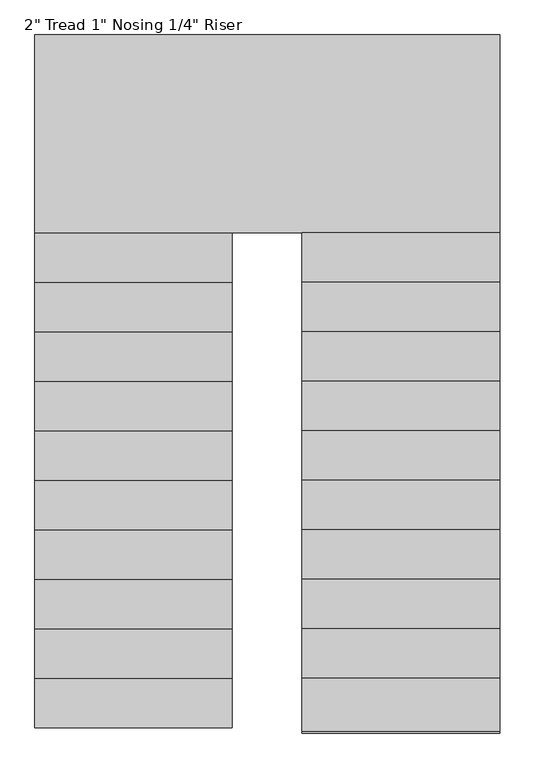
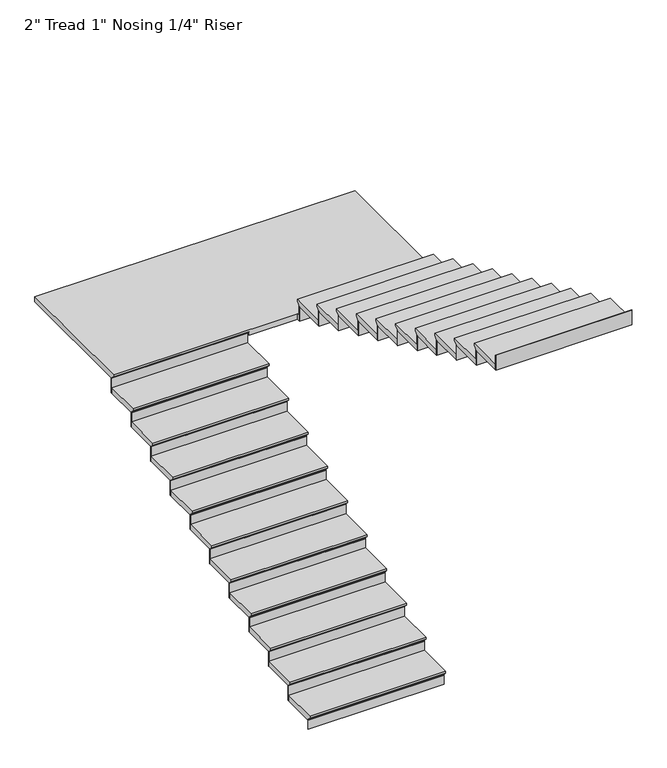
"""IFC4 building model written with IfcOpenShell, lengths in millimetres: stair flight geometry."""

from ifc_helpers import new_model, si_unit, origin, place, context, project, spatial, faceted_brep, source, transform, mapped, element, save


def stair_flight_66ca282f(model_context):
    return source(origin(), model_context, "Body", "Brep", [
        faceted_brep([(-629.5987998, 3364.6067329, 28923.0954545), (-629.5987998, 3364.6067329, 28942.1454545), (-1845.5417538, 3364.6067329, 28942.1454545), (-1845.5417538, 3364.6067329, 28923.0954545), (-629.5987998, 3390.0067329, 28897.6954545), (-1845.5417538, 3390.0067329, 28897.6954545), (-629.5987998, 3694.8067329, 28942.1454545), (-1845.5417538, 3694.8067329, 28942.1454545), (-1845.5417538, 3390.0067329, 28891.3454545), (-1845.5417538, 3694.8067329, 28891.3454545), (-629.5987998, 3694.8067329, 28891.3454545), (-629.5987998, 3390.0067329, 28891.3454545)], [[[0, 1, 2, 3]], [[4, 0, 3, 5]], [[2, 1, 6, 7]], [[8, 9, 10, 11]], [[2, 7, 9, 8, 5, 3]], [[8, 11, 4, 5]], [[6, 1, 0, 4, 11, 10]], [[7, 6, 10, 9]]]),
        faceted_brep([(-629.5987998, 3390.0067329, 28891.3454545), (-629.5987998, 3390.0067329, 28803.6), (-629.5987998, 3396.3567329, 28803.6), (-629.5987998, 3396.3567329, 28891.3454545), (-1845.5417538, 3390.0067329, 28891.3454545), (-1845.5417538, 3396.3567329, 28891.3454545), (-1845.5417538, 3396.3567329, 28803.6), (-1845.5417538, 3390.0067329, 28803.6)], [[[0, 1, 2, 3]], [[4, 5, 6, 7]], [[1, 0, 4, 7]], [[2, 1, 7, 6]], [[3, 2, 6, 5]], [[0, 3, 5, 4]]]),
        faceted_brep([(-629.5987998, 3694.8067329, 29029.8909091), (-629.5987998, 3694.8067329, 28891.3454545), (-629.5987998, 3701.1567329, 28891.3454545), (-629.5987998, 3701.1567329, 29029.8909091), (-1845.5417538, 3694.8067329, 29029.8909091), (-1845.5417538, 3701.1567329, 29029.8909091), (-1845.5417538, 3701.1567329, 28891.3454545), (-1845.5417538, 3694.8067329, 28891.3454545)], [[[0, 1, 2, 3]], [[4, 5, 6, 7]], [[1, 0, 4, 7]], [[2, 1, 7, 6]], [[3, 2, 6, 5]], [[0, 3, 5, 4]]]),
        faceted_brep([(-1845.5417538, 3669.4067329, 29080.6909091), (-629.5987998, 3669.4067329, 29080.6909091), (-629.5987998, 3999.6067329, 29080.6909091), (-1845.5417538, 3999.6067329, 29080.6909091), (-1845.5417538, 3694.8067329, 29029.8909091), (-1845.5417538, 3999.6067329, 29029.8909091), (-629.5987998, 3999.6067329, 29029.8909091), (-629.5987998, 3694.8067329, 29029.8909091), (-1845.5417538, 3694.8067329, 29036.2409091), (-1845.5417538, 3669.4067329, 29061.6409091), (-629.5987998, 3694.8067329, 29036.2409091), (-629.5987998, 3669.4067329, 29061.6409091)], [[[0, 1, 2, 3]], [[4, 5, 6, 7]], [[0, 3, 5, 4, 8, 9]], [[4, 7, 10, 8]], [[2, 1, 11, 10, 7, 6]], [[3, 2, 6, 5]], [[11, 1, 0, 9]], [[10, 11, 9, 8]]]),
        faceted_brep([(-629.5987998, 3999.6067329, 29168.4363636), (-629.5987998, 3999.6067329, 29029.8909091), (-629.5987998, 4005.9567329, 29029.8909091), (-629.5987998, 4005.9567329, 29168.4363636), (-1845.5417538, 3999.6067329, 29168.4363636), (-1845.5417538, 4005.9567329, 29168.4363636), (-1845.5417538, 4005.9567329, 29029.8909091), (-1845.5417538, 3999.6067329, 29029.8909091)], [[[0, 1, 2, 3]], [[4, 5, 6, 7]], [[1, 0, 4, 7]], [[2, 1, 7, 6]], [[3, 2, 6, 5]], [[0, 3, 5, 4]]]),
        faceted_brep([(-1845.5417538, 3974.2067329, 29219.2363636), (-629.5987998, 3974.2067329, 29219.2363636), (-629.5987998, 4304.4067329, 29219.2363636), (-1845.5417538, 4304.4067329, 29219.2363636), (-1845.5417538, 3999.6067329, 29168.4363636), (-1845.5417538, 4304.4067329, 29168.4363636), (-629.5987998, 4304.4067329, 29168.4363636), (-629.5987998, 3999.6067329, 29168.4363636), (-1845.5417538, 3999.6067329, 29174.7863636), (-1845.5417538, 3974.2067329, 29200.1863636), (-629.5987998, 3999.6067329, 29174.7863636), (-629.5987998, 3974.2067329, 29200.1863636)], [[[0, 1, 2, 3]], [[4, 5, 6, 7]], [[0, 3, 5, 4, 8, 9]], [[4, 7, 10, 8]], [[2, 1, 11, 10, 7, 6]], [[3, 2, 6, 5]], [[11, 1, 0, 9]], [[10, 11, 9, 8]]]),
        faceted_brep([(-629.5987998, 4304.4067329, 29306.9818182), (-629.5987998, 4304.4067329, 29168.4363636), (-629.5987998, 4310.7567329, 29168.4363636), (-629.5987998, 4310.7567329, 29306.9818182), (-1845.5417538, 4304.4067329, 29306.9818182), (-1845.5417538, 4310.7567329, 29306.9818182), (-1845.5417538, 4310.7567329, 29168.4363636), (-1845.5417538, 4304.4067329, 29168.4363636)], [[[0, 1, 2, 3]], [[4, 5, 6, 7]], [[1, 0, 4, 7]], [[2, 1, 7, 6]], [[3, 2, 6, 5]], [[0, 3, 5, 4]]]),
        faceted_brep([(-1845.5417538, 4279.0067329, 29357.7818182), (-629.5987998, 4279.0067329, 29357.7818182), (-629.5987998, 4609.2067329, 29357.7818182), (-1845.5417538, 4609.2067329, 29357.7818182), (-1845.5417538, 4304.4067329, 29306.9818182), (-1845.5417538, 4609.2067329, 29306.9818182), (-629.5987998, 4609.2067329, 29306.9818182), (-629.5987998, 4304.4067329, 29306.9818182), (-1845.5417538, 4304.4067329, 29313.3318182), (-1845.5417538, 4279.0067329, 29338.7318182), (-629.5987998, 4304.4067329, 29313.3318182), (-629.5987998, 4279.0067329, 29338.7318182)], [[[0, 1, 2, 3]], [[4, 5, 6, 7]], [[0, 3, 5, 4, 8, 9]], [[4, 7, 10, 8]], [[2, 1, 11, 10, 7, 6]], [[3, 2, 6, 5]], [[11, 1, 0, 9]], [[10, 11, 9, 8]]]),
        faceted_brep([(-629.5987998, 4609.2067329, 29445.5272727), (-629.5987998, 4609.2067329, 29306.9818182), (-629.5987998, 4615.5567329, 29306.9818182), (-629.5987998, 4615.5567329, 29445.5272727), (-1845.5417538, 4609.2067329, 29445.5272727), (-1845.5417538, 4615.5567329, 29445.5272727), (-1845.5417538, 4615.5567329, 29306.9818182), (-1845.5417538, 4609.2067329, 29306.9818182)], [[[0, 1, 2, 3]], [[4, 5, 6, 7]], [[1, 0, 4, 7]], [[2, 1, 7, 6]], [[3, 2, 6, 5]], [[0, 3, 5, 4]]]),
        faceted_brep([(-1845.5417538, 4583.8067329, 29496.3272727), (-629.5987998, 4583.8067329, 29496.3272727), (-629.5987998, 4914.0067329, 29496.3272727), (-1845.5417538, 4914.0067329, 29496.3272727), (-1845.5417538, 4609.2067329, 29445.5272727), (-1845.5417538, 4914.0067329, 29445.5272727), (-629.5987998, 4914.0067329, 29445.5272727), (-629.5987998, 4609.2067329, 29445.5272727), (-1845.5417538, 4609.2067329, 29451.8772727), (-1845.5417538, 4583.8067329, 29477.2772727), (-629.5987998, 4609.2067329, 29451.8772727), (-629.5987998, 4583.8067329, 29477.2772727)], [[[0, 1, 2, 3]], [[4, 5, 6, 7]], [[0, 3, 5, 4, 8, 9]], [[4, 7, 10, 8]], [[2, 1, 11, 10, 7, 6]], [[3, 2, 6, 5]], [[11, 1, 0, 9]], [[10, 11, 9, 8]]]),
        faceted_brep([(-629.5987998, 4914.0067329, 29584.0727273), (-629.5987998, 4914.0067329, 29445.5272727), (-629.5987998, 4920.3567329, 29445.5272727), (-629.5987998, 4920.3567329, 29584.0727273), (-1845.5417538, 4914.0067329, 29584.0727273), (-1845.5417538, 4920.3567329, 29584.0727273), (-1845.5417538, 4920.3567329, 29445.5272727), (-1845.5417538, 4914.0067329, 29445.5272727)], [[[0, 1, 2, 3]], [[4, 5, 6, 7]], [[1, 0, 4, 7]], [[2, 1, 7, 6]], [[3, 2, 6, 5]], [[0, 3, 5, 4]]]),
        faceted_brep([(-1845.5417538, 4888.6067329, 29634.8727273), (-629.5987998, 4888.6067329, 29634.8727273), (-629.5987998, 5218.8067329, 29634.8727273), (-1845.5417538, 5218.8067329, 29634.8727273), (-1845.5417538, 4914.0067329, 29584.0727273), (-1845.5417538, 5218.8067329, 29584.0727273), (-629.5987998, 5218.8067329, 29584.0727273), (-629.5987998, 4914.0067329, 29584.0727273), (-1845.5417538, 4914.0067329, 29590.4227273), (-1845.5417538, 4888.6067329, 29615.8227273), (-629.5987998, 4914.0067329, 29590.4227273), (-629.5987998, 4888.6067329, 29615.8227273)], [[[0, 1, 2, 3]], [[4, 5, 6, 7]], [[0, 3, 5, 4, 8, 9]], [[4, 7, 10, 8]], [[2, 1, 11, 10, 7, 6]], [[3, 2, 6, 5]], [[11, 1, 0, 9]], [[10, 11, 9, 8]]]),
        faceted_brep([(-629.5987998, 5218.8067329, 29722.6181818), (-629.5987998, 5218.8067329, 29584.0727273), (-629.5987998, 5225.1567329, 29584.0727273), (-629.5987998, 5225.1567329, 29722.6181818), (-1845.5417538, 5218.8067329, 29722.6181818), (-1845.5417538, 5225.1567329, 29722.6181818), (-1845.5417538, 5225.1567329, 29584.0727273), (-1845.5417538, 5218.8067329, 29584.0727273)], [[[0, 1, 2, 3]], [[4, 5, 6, 7]], [[1, 0, 4, 7]], [[2, 1, 7, 6]], [[3, 2, 6, 5]], [[0, 3, 5, 4]]]),
        faceted_brep([(-1845.5417538, 5193.4067329, 29773.4181818), (-629.5987998, 5193.4067329, 29773.4181818), (-629.5987998, 5523.6067329, 29773.4181818), (-1845.5417538, 5523.6067329, 29773.4181818), (-1845.5417538, 5218.8067329, 29722.6181818), (-1845.5417538, 5523.6067329, 29722.6181818), (-629.5987998, 5523.6067329, 29722.6181818), (-629.5987998, 5218.8067329, 29722.6181818), (-1845.5417538, 5218.8067329, 29728.9681818), (-1845.5417538, 5193.4067329, 29754.3681818), (-629.5987998, 5218.8067329, 29728.9681818), (-629.5987998, 5193.4067329, 29754.3681818)], [[[0, 1, 2, 3]], [[4, 5, 6, 7]], [[0, 3, 5, 4, 8, 9]], [[4, 7, 10, 8]], [[2, 1, 11, 10, 7, 6]], [[3, 2, 6, 5]], [[11, 1, 0, 9]], [[10, 11, 9, 8]]]),
        faceted_brep([(-629.5987998, 5523.6067329, 29861.1636364), (-629.5987998, 5523.6067329, 29722.6181818), (-629.5987998, 5529.9567329, 29722.6181818), (-629.5987998, 5529.9567329, 29861.1636364), (-1845.5417538, 5523.6067329, 29861.1636364), (-1845.5417538, 5529.9567329, 29861.1636364), (-1845.5417538, 5529.9567329, 29722.6181818), (-1845.5417538, 5523.6067329, 29722.6181818)], [[[0, 1, 2, 3]], [[4, 5, 6, 7]], [[1, 0, 4, 7]], [[2, 1, 7, 6]], [[3, 2, 6, 5]], [[0, 3, 5, 4]]]),
        faceted_brep([(-1845.5417538, 5498.2067329, 29911.9636364), (-629.5987998, 5498.2067329, 29911.9636364), (-629.5987998, 5828.4067329, 29911.9636364), (-1845.5417538, 5828.4067329, 29911.9636364), (-1845.5417538, 5523.6067329, 29861.1636364), (-1845.5417538, 5828.4067329, 29861.1636364), (-629.5987998, 5828.4067329, 29861.1636364), (-629.5987998, 5523.6067329, 29861.1636364), (-1845.5417538, 5523.6067329, 29867.5136364), (-1845.5417538, 5498.2067329, 29892.9136364), (-629.5987998, 5523.6067329, 29867.5136364), (-629.5987998, 5498.2067329, 29892.9136364)], [[[0, 1, 2, 3]], [[4, 5, 6, 7]], [[0, 3, 5, 4, 8, 9]], [[4, 7, 10, 8]], [[2, 1, 11, 10, 7, 6]], [[3, 2, 6, 5]], [[11, 1, 0, 9]], [[10, 11, 9, 8]]]),
        faceted_brep([(-629.5987998, 5828.4067329, 29999.7090909), (-629.5987998, 5828.4067329, 29861.1636364), (-629.5987998, 5834.7567329, 29861.1636364), (-629.5987998, 5834.7567329, 29999.7090909), (-1845.5417538, 5828.4067329, 29999.7090909), (-1845.5417538, 5834.7567329, 29999.7090909), (-1845.5417538, 5834.7567329, 29861.1636364), (-1845.5417538, 5828.4067329, 29861.1636364)], [[[0, 1, 2, 3]], [[4, 5, 6, 7]], [[1, 0, 4, 7]], [[2, 1, 7, 6]], [[3, 2, 6, 5]], [[0, 3, 5, 4]]]),
        faceted_brep([(-1845.5417538, 5803.0067329, 30050.5090909), (-629.5987998, 5803.0067329, 30050.5090909), (-629.5987998, 6133.2067329, 30050.5090909), (-1845.5417538, 6133.2067329, 30050.5090909), (-1845.5417538, 5828.4067329, 29999.7090909), (-1845.5417538, 6133.2067329, 29999.7090909), (-629.5987998, 6133.2067329, 29999.7090909), (-629.5987998, 5828.4067329, 29999.7090909), (-1845.5417538, 5828.4067329, 30006.0590909), (-1845.5417538, 5803.0067329, 30031.4590909), (-629.5987998, 5828.4067329, 30006.0590909), (-629.5987998, 5803.0067329, 30031.4590909)], [[[0, 1, 2, 3]], [[4, 5, 6, 7]], [[0, 3, 5, 4, 8, 9]], [[4, 7, 10, 8]], [[2, 1, 11, 10, 7, 6]], [[3, 2, 6, 5]], [[11, 1, 0, 9]], [[10, 11, 9, 8]]]),
        faceted_brep([(-629.5987998, 6133.2067329, 30138.2545455), (-629.5987998, 6133.2067329, 29999.7090909), (-629.5987998, 6139.5567329, 29999.7090909), (-629.5987998, 6139.5567329, 30138.2545455), (-1845.5417538, 6133.2067329, 30138.2545455), (-1845.5417538, 6139.5567329, 30138.2545455), (-1845.5417538, 6139.5567329, 29999.7090909), (-1845.5417538, 6133.2067329, 29999.7090909)], [[[0, 1, 2, 3]], [[4, 5, 6, 7]], [[1, 0, 4, 7]], [[2, 1, 7, 6]], [[3, 2, 6, 5]], [[0, 3, 5, 4]]]),
        faceted_brep([(-1845.5417538, 6107.8067329, 30189.0545455), (-629.5987998, 6107.8067329, 30189.0545455), (-629.5987998, 6438.0067329, 30189.0545455), (-1845.5417538, 6438.0067329, 30189.0545455), (-1845.5417538, 6133.2067329, 30138.2545455), (-1845.5417538, 6438.0067329, 30138.2545455), (-629.5987998, 6438.0067329, 30138.2545455), (-629.5987998, 6133.2067329, 30138.2545455), (-1845.5417538, 6133.2067329, 30144.6045455), (-1845.5417538, 6107.8067329, 30170.0045455), (-629.5987998, 6133.2067329, 30144.6045455), (-629.5987998, 6107.8067329, 30170.0045455)], [[[0, 1, 2, 3]], [[4, 5, 6, 7]], [[0, 3, 5, 4, 8, 9]], [[4, 7, 10, 8]], [[2, 1, 11, 10, 7, 6]], [[3, 2, 6, 5]], [[11, 1, 0, 9]], [[10, 11, 9, 8]]]),
        faceted_brep([(-629.5987998, 6438.0067329, 30276.8), (-629.5987998, 6438.0067329, 30138.2545455), (-629.5987998, 6444.3567329, 30138.2545455), (-629.5987998, 6444.3567329, 30276.8), (-1845.5417538, 6438.0067329, 30276.8), (-1845.5417538, 6444.3567329, 30276.8), (-1845.5417538, 6444.3567329, 30138.2545455), (-1845.5417538, 6438.0067329, 30138.2545455)], [[[0, 1, 2, 3]], [[4, 5, 6, 7]], [[1, 0, 4, 7]], [[2, 1, 7, 6]], [[3, 2, 6, 5]], [[0, 3, 5, 4]]]),
        faceted_brep([(1021.4012085, 6387.2067329, 30327.6), (1021.4012085, 7631.8067329, 30327.6), (-1845.5417538, 7631.8067329, 30327.6), (-1845.5417538, 6412.6067329, 30327.6), (-197.7987915, 6412.6067329, 30327.6), (-197.7987915, 6387.2067329, 30327.6), (1021.4012085, 7631.8067329, 30276.8), (1021.4012085, 6387.2067329, 30276.8), (-197.7987915, 6387.2067329, 30276.8), (-197.7987915, 6412.6067329, 30276.8), (-629.5987998, 6412.6067329, 30276.8), (-629.5987998, 6438.0067329, 30276.8), (-1845.5417538, 6438.0067329, 30276.8), (-1845.5417538, 7631.8067329, 30276.8), (-629.5987998, 6438.0067329, 30283.15), (-1845.5417538, 6438.0067329, 30283.15), (-1845.5417538, 6412.6067329, 30308.55), (-629.5987998, 6412.6067329, 30308.55)], [[[0, 1, 2, 3, 4, 5]], [[6, 7, 8, 9, 10, 11, 12, 13]], [[1, 0, 7, 6]], [[2, 1, 6, 13]], [[12, 11, 14, 15]], [[4, 3, 16, 17, 10, 9]], [[5, 4, 9, 8]], [[0, 5, 8, 7]], [[16, 15, 14, 17]], [[3, 2, 13, 12, 15, 16]], [[11, 10, 17, 14]]]),
        faceted_brep([(-197.7987915, 6387.2067329, 30415.3454545), (-197.7987915, 6387.2067329, 30276.8), (-197.7987915, 6380.8567329, 30276.8), (-197.7987915, 6380.8567329, 30415.3454545), (1021.4012085, 6387.2067329, 30415.3454545), (1021.4012085, 6380.8567329, 30415.3454545), (1021.4012085, 6380.8567329, 30276.8), (1021.4012085, 6387.2067329, 30276.8)], [[[0, 1, 2, 3]], [[4, 5, 6, 7]], [[1, 0, 4, 7]], [[2, 1, 7, 6]], [[3, 2, 6, 5]], [[0, 3, 5, 4]]]),
        faceted_brep([(1021.4012085, 6412.6067329, 30466.1454545), (-197.7987915, 6412.6067329, 30466.1454545), (-197.7987915, 6082.4067329, 30466.1454545), (1021.4012085, 6082.4067329, 30466.1454545), (1021.4012085, 6387.2067329, 30415.3454545), (1021.4012085, 6082.4067329, 30415.3454545), (-197.7987915, 6082.4067329, 30415.3454545), (-197.7987915, 6387.2067329, 30415.3454545), (1021.4012085, 6387.2067329, 30421.6954545), (1021.4012085, 6412.6067329, 30447.0954545), (-197.7987915, 6387.2067329, 30421.6954545), (-197.7987915, 6412.6067329, 30447.0954545)], [[[0, 1, 2, 3]], [[4, 5, 6, 7]], [[0, 3, 5, 4, 8, 9]], [[4, 7, 10, 8]], [[2, 1, 11, 10, 7, 6]], [[3, 2, 6, 5]], [[11, 1, 0, 9]], [[10, 11, 9, 8]]]),
        faceted_brep([(-197.7987915, 6082.4067329, 30553.8909091), (-197.7987915, 6082.4067329, 30415.3454545), (-197.7987915, 6076.0567329, 30415.3454545), (-197.7987915, 6076.0567329, 30553.8909091), (1021.4012085, 6082.4067329, 30553.8909091), (1021.4012085, 6076.0567329, 30553.8909091), (1021.4012085, 6076.0567329, 30415.3454545), (1021.4012085, 6082.4067329, 30415.3454545)], [[[0, 1, 2, 3]], [[4, 5, 6, 7]], [[1, 0, 4, 7]], [[2, 1, 7, 6]], [[3, 2, 6, 5]], [[0, 3, 5, 4]]]),
        faceted_brep([(1021.4012085, 6107.8067329, 30604.6909091), (-197.7987915, 6107.8067329, 30604.6909091), (-197.7987915, 5777.6067329, 30604.6909091), (1021.4012085, 5777.6067329, 30604.6909091), (1021.4012085, 6082.4067329, 30553.8909091), (1021.4012085, 5777.6067329, 30553.8909091), (-197.7987915, 5777.6067329, 30553.8909091), (-197.7987915, 6082.4067329, 30553.8909091), (1021.4012085, 6082.4067329, 30560.2409091), (1021.4012085, 6107.8067329, 30585.6409091), (-197.7987915, 6082.4067329, 30560.2409091), (-197.7987915, 6107.8067329, 30585.6409091)], [[[0, 1, 2, 3]], [[4, 5, 6, 7]], [[0, 3, 5, 4, 8, 9]], [[4, 7, 10, 8]], [[2, 1, 11, 10, 7, 6]], [[3, 2, 6, 5]], [[11, 1, 0, 9]], [[10, 11, 9, 8]]]),
        faceted_brep([(-197.7987915, 5777.6067329, 30692.4363636), (-197.7987915, 5777.6067329, 30553.8909091), (-197.7987915, 5771.2567329, 30553.8909091), (-197.7987915, 5771.2567329, 30692.4363636), (1021.4012085, 5777.6067329, 30692.4363636), (1021.4012085, 5771.2567329, 30692.4363636), (1021.4012085, 5771.2567329, 30553.8909091), (1021.4012085, 5777.6067329, 30553.8909091)], [[[0, 1, 2, 3]], [[4, 5, 6, 7]], [[1, 0, 4, 7]], [[2, 1, 7, 6]], [[3, 2, 6, 5]], [[0, 3, 5, 4]]]),
        faceted_brep([(1021.4012085, 5803.0067329, 30743.2363636), (-197.7987915, 5803.0067329, 30743.2363636), (-197.7987915, 5472.8067329, 30743.2363636), (1021.4012085, 5472.8067329, 30743.2363636), (1021.4012085, 5777.6067329, 30692.4363636), (1021.4012085, 5472.8067329, 30692.4363636), (-197.7987915, 5472.8067329, 30692.4363636), (-197.7987915, 5777.6067329, 30692.4363636), (1021.4012085, 5777.6067329, 30698.7863636), (1021.4012085, 5803.0067329, 30724.1863636), (-197.7987915, 5777.6067329, 30698.7863636), (-197.7987915, 5803.0067329, 30724.1863636)], [[[0, 1, 2, 3]], [[4, 5, 6, 7]], [[0, 3, 5, 4, 8, 9]], [[4, 7, 10, 8]], [[2, 1, 11, 10, 7, 6]], [[3, 2, 6, 5]], [[11, 1, 0, 9]], [[10, 11, 9, 8]]]),
        faceted_brep([(-197.7987915, 5472.8067329, 30830.9818182), (-197.7987915, 5472.8067329, 30692.4363636), (-197.7987915, 5466.4567329, 30692.4363636), (-197.7987915, 5466.4567329, 30830.9818182), (1021.4012085, 5472.8067329, 30830.9818182), (1021.4012085, 5466.4567329, 30830.9818182), (1021.4012085, 5466.4567329, 30692.4363636), (1021.4012085, 5472.8067329, 30692.4363636)], [[[0, 1, 2, 3]], [[4, 5, 6, 7]], [[1, 0, 4, 7]], [[2, 1, 7, 6]], [[3, 2, 6, 5]], [[0, 3, 5, 4]]]),
        faceted_brep([(1021.4012085, 5498.2067329, 30881.7818182), (-197.7987915, 5498.2067329, 30881.7818182), (-197.7987915, 5168.0067329, 30881.7818182), (1021.4012085, 5168.0067329, 30881.7818182), (1021.4012085, 5472.8067329, 30830.9818182), (1021.4012085, 5168.0067329, 30830.9818182), (-197.7987915, 5168.0067329, 30830.9818182), (-197.7987915, 5472.8067329, 30830.9818182), (1021.4012085, 5472.8067329, 30837.3318182), (1021.4012085, 5498.2067329, 30862.7318182), (-197.7987915, 5472.8067329, 30837.3318182), (-197.7987915, 5498.2067329, 30862.7318182)], [[[0, 1, 2, 3]], [[4, 5, 6, 7]], [[0, 3, 5, 4, 8, 9]], [[4, 7, 10, 8]], [[2, 1, 11, 10, 7, 6]], [[3, 2, 6, 5]], [[11, 1, 0, 9]], [[10, 11, 9, 8]]]),
        faceted_brep([(-197.7987915, 5168.0067329, 30969.5272727), (-197.7987915, 5168.0067329, 30830.9818182), (-197.7987915, 5161.6567329, 30830.9818182), (-197.7987915, 5161.6567329, 30969.5272727), (1021.4012085, 5168.0067329, 30969.5272727), (1021.4012085, 5161.6567329, 30969.5272727), (1021.4012085, 5161.6567329, 30830.9818182), (1021.4012085, 5168.0067329, 30830.9818182)], [[[0, 1, 2, 3]], [[4, 5, 6, 7]], [[1, 0, 4, 7]], [[2, 1, 7, 6]], [[3, 2, 6, 5]], [[0, 3, 5, 4]]]),
        faceted_brep([(1021.4012085, 5193.4067329, 31020.3272727), (-197.7987915, 5193.4067329, 31020.3272727), (-197.7987915, 4863.2067329, 31020.3272727), (1021.4012085, 4863.2067329, 31020.3272727), (1021.4012085, 5168.0067329, 30969.5272727), (1021.4012085, 4863.2067329, 30969.5272727), (-197.7987915, 4863.2067329, 30969.5272727), (-197.7987915, 5168.0067329, 30969.5272727), (1021.4012085, 5168.0067329, 30975.8772727), (1021.4012085, 5193.4067329, 31001.2772727), (-197.7987915, 5168.0067329, 30975.8772727), (-197.7987915, 5193.4067329, 31001.2772727)], [[[0, 1, 2, 3]], [[4, 5, 6, 7]], [[0, 3, 5, 4, 8, 9]], [[4, 7, 10, 8]], [[2, 1, 11, 10, 7, 6]], [[3, 2, 6, 5]], [[11, 1, 0, 9]], [[10, 11, 9, 8]]]),
        faceted_brep([(-197.7987915, 4863.2067329, 31108.0727273), (-197.7987915, 4863.2067329, 30969.5272727), (-197.7987915, 4856.8567329, 30969.5272727), (-197.7987915, 4856.8567329, 31108.0727273), (1021.4012085, 4863.2067329, 31108.0727273), (1021.4012085, 4856.8567329, 31108.0727273), (1021.4012085, 4856.8567329, 30969.5272727), (1021.4012085, 4863.2067329, 30969.5272727)], [[[0, 1, 2, 3]], [[4, 5, 6, 7]], [[1, 0, 4, 7]], [[2, 1, 7, 6]], [[3, 2, 6, 5]], [[0, 3, 5, 4]]]),
        faceted_brep([(1021.4012085, 4888.6067329, 31158.8727273), (-197.7987915, 4888.6067329, 31158.8727273), (-197.7987915, 4558.4067329, 31158.8727273), (1021.4012085, 4558.4067329, 31158.8727273), (1021.4012085, 4863.2067329, 31108.0727273), (1021.4012085, 4558.4067329, 31108.0727273), (-197.7987915, 4558.4067329, 31108.0727273), (-197.7987915, 4863.2067329, 31108.0727273), (1021.4012085, 4863.2067329, 31114.4227273), (1021.4012085, 4888.6067329, 31139.8227273), (-197.7987915, 4863.2067329, 31114.4227273), (-197.7987915, 4888.6067329, 31139.8227273)], [[[0, 1, 2, 3]], [[4, 5, 6, 7]], [[0, 3, 5, 4, 8, 9]], [[4, 7, 10, 8]], [[2, 1, 11, 10, 7, 6]], [[3, 2, 6, 5]], [[11, 1, 0, 9]], [[10, 11, 9, 8]]]),
        faceted_brep([(-197.7987915, 4558.4067329, 31246.6181818), (-197.7987915, 4558.4067329, 31108.0727273), (-197.7987915, 4552.0567329, 31108.0727273), (-197.7987915, 4552.0567329, 31246.6181818), (1021.4012085, 4558.4067329, 31246.6181818), (1021.4012085, 4552.0567329, 31246.6181818), (1021.4012085, 4552.0567329, 31108.0727273), (1021.4012085, 4558.4067329, 31108.0727273)], [[[0, 1, 2, 3]], [[4, 5, 6, 7]], [[1, 0, 4, 7]], [[2, 1, 7, 6]], [[3, 2, 6, 5]], [[0, 3, 5, 4]]]),
        faceted_brep([(1021.4012085, 4583.8067329, 31297.4181818), (-197.7987915, 4583.8067329, 31297.4181818), (-197.7987915, 4253.6067329, 31297.4181818), (1021.4012085, 4253.6067329, 31297.4181818), (1021.4012085, 4558.4067329, 31246.6181818), (1021.4012085, 4253.6067329, 31246.6181818), (-197.7987915, 4253.6067329, 31246.6181818), (-197.7987915, 4558.4067329, 31246.6181818), (1021.4012085, 4558.4067329, 31252.9681818), (1021.4012085, 4583.8067329, 31278.3681818), (-197.7987915, 4558.4067329, 31252.9681818), (-197.7987915, 4583.8067329, 31278.3681818)], [[[0, 1, 2, 3]], [[4, 5, 6, 7]], [[0, 3, 5, 4, 8, 9]], [[4, 7, 10, 8]], [[2, 1, 11, 10, 7, 6]], [[3, 2, 6, 5]], [[11, 1, 0, 9]], [[10, 11, 9, 8]]]),
        faceted_brep([(-197.7987915, 4253.6067329, 31385.1636364), (-197.7987915, 4253.6067329, 31246.6181818), (-197.7987915, 4247.2567329, 31246.6181818), (-197.7987915, 4247.2567329, 31385.1636364), (1021.4012085, 4253.6067329, 31385.1636364), (1021.4012085, 4247.2567329, 31385.1636364), (1021.4012085, 4247.2567329, 31246.6181818), (1021.4012085, 4253.6067329, 31246.6181818)], [[[0, 1, 2, 3]], [[4, 5, 6, 7]], [[1, 0, 4, 7]], [[2, 1, 7, 6]], [[3, 2, 6, 5]], [[0, 3, 5, 4]]]),
        faceted_brep([(1021.4012085, 4279.0067329, 31435.9636364), (-197.7987915, 4279.0067329, 31435.9636364), (-197.7987915, 3948.8067329, 31435.9636364), (1021.4012085, 3948.8067329, 31435.9636364), (1021.4012085, 4253.6067329, 31385.1636364), (1021.4012085, 3948.8067329, 31385.1636364), (-197.7987915, 3948.8067329, 31385.1636364), (-197.7987915, 4253.6067329, 31385.1636364), (1021.4012085, 4253.6067329, 31391.5136364), (1021.4012085, 4279.0067329, 31416.9136364), (-197.7987915, 4253.6067329, 31391.5136364), (-197.7987915, 4279.0067329, 31416.9136364)], [[[0, 1, 2, 3]], [[4, 5, 6, 7]], [[0, 3, 5, 4, 8, 9]], [[4, 7, 10, 8]], [[2, 1, 11, 10, 7, 6]], [[3, 2, 6, 5]], [[11, 1, 0, 9]], [[10, 11, 9, 8]]]),
        faceted_brep([(-197.7987915, 3948.8067329, 31523.7090909), (-197.7987915, 3948.8067329, 31385.1636364), (-197.7987915, 3942.4567329, 31385.1636364), (-197.7987915, 3942.4567329, 31523.7090909), (1021.4012085, 3948.8067329, 31523.7090909), (1021.4012085, 3942.4567329, 31523.7090909), (1021.4012085, 3942.4567329, 31385.1636364), (1021.4012085, 3948.8067329, 31385.1636364)], [[[0, 1, 2, 3]], [[4, 5, 6, 7]], [[1, 0, 4, 7]], [[2, 1, 7, 6]], [[3, 2, 6, 5]], [[0, 3, 5, 4]]]),
        faceted_brep([(1021.4012085, 3974.2067329, 31574.5090909), (-197.7987915, 3974.2067329, 31574.5090909), (-197.7987915, 3644.0067329, 31574.5090909), (1021.4012085, 3644.0067329, 31574.5090909), (1021.4012085, 3948.8067329, 31523.7090909), (1021.4012085, 3644.0067329, 31523.7090909), (-197.7987915, 3644.0067329, 31523.7090909), (-197.7987915, 3948.8067329, 31523.7090909), (1021.4012085, 3948.8067329, 31530.0590909), (1021.4012085, 3974.2067329, 31555.4590909), (-197.7987915, 3948.8067329, 31530.0590909), (-197.7987915, 3974.2067329, 31555.4590909)], [[[0, 1, 2, 3]], [[4, 5, 6, 7]], [[0, 3, 5, 4, 8, 9]], [[4, 7, 10, 8]], [[2, 1, 11, 10, 7, 6]], [[3, 2, 6, 5]], [[11, 1, 0, 9]], [[10, 11, 9, 8]]]),
        faceted_brep([(-197.7987915, 3644.0067329, 31662.2545455), (-197.7987915, 3644.0067329, 31523.7090909), (-197.7987915, 3637.6567329, 31523.7090909), (-197.7987915, 3637.6567329, 31662.2545455), (1021.4012085, 3644.0067329, 31662.2545455), (1021.4012085, 3637.6567329, 31662.2545455), (1021.4012085, 3637.6567329, 31523.7090909), (1021.4012085, 3644.0067329, 31523.7090909)], [[[0, 1, 2, 3]], [[4, 5, 6, 7]], [[1, 0, 4, 7]], [[2, 1, 7, 6]], [[3, 2, 6, 5]], [[0, 3, 5, 4]]]),
        faceted_brep([(-197.7987915, 3339.2067329, 31800.8), (-197.7987915, 3339.2067329, 31662.2545455), (-197.7987915, 3332.8567329, 31662.2545455), (-197.7987915, 3332.8567329, 31800.8), (1021.4012085, 3339.2067329, 31800.8), (1021.4012085, 3332.8567329, 31800.8), (1021.4012085, 3332.8567329, 31662.2545455), (1021.4012085, 3339.2067329, 31662.2545455)], [[[0, 1, 2, 3]], [[4, 5, 6, 7]], [[1, 0, 4, 7]], [[2, 1, 7, 6]], [[3, 2, 6, 5]], [[0, 3, 5, 4]]]),
        faceted_brep([(1021.4012085, 3669.4067329, 31713.0545455), (-197.7987915, 3669.4067329, 31713.0545455), (-197.7987915, 3339.2067329, 31713.0545455), (1021.4012085, 3339.2067329, 31713.0545455), (1021.4012085, 3644.0067329, 31662.2545455), (1021.4012085, 3339.2067329, 31662.2545455), (-197.7987915, 3339.2067329, 31662.2545455), (-197.7987915, 3644.0067329, 31662.2545455), (1021.4012085, 3644.0067329, 31668.6045455), (1021.4012085, 3669.4067329, 31694.0045455), (-197.7987915, 3644.0067329, 31668.6045455), (-197.7987915, 3669.4067329, 31694.0045455)], [[[0, 1, 2, 3]], [[4, 5, 6, 7]], [[0, 3, 5, 4, 8, 9]], [[4, 7, 10, 8]], [[2, 1, 11, 10, 7, 6]], [[3, 2, 6, 5]], [[11, 1, 0, 9]], [[10, 11, 9, 8]]]),
    ])


if __name__ == "__main__":
    model = new_model("IFC4")
    model_context = context("Model", 3, world=origin())
    ifc_project = project(units=[si_unit("LENGTHUNIT", "METRE", prefix="MILLI")], contexts=[model_context])
    site = spatial("IfcSite", under=ifc_project)
    building = spatial("IfcBuilding", under=site)
    placement = place(None, origin())
    stair_flight_shape = stair_flight_66ca282f(model_context)
    element("IfcStairFlight", 1, ObjectType="2\" Tread 1\" Nosing 1/4\" Riser", at=placement, inside=building, context=model_context, shape_type="MappedRepresentation", body=[
        mapped(stair_flight_shape, transform((0.0, 0.0, 0.0), x_axis=(1.0, 0.0, 0.0), y_axis=(0.0, 1.0, 0.0), z_axis=(0.0, 0.0, 1.0))),
    ])
    save(model, "model.ifc")
